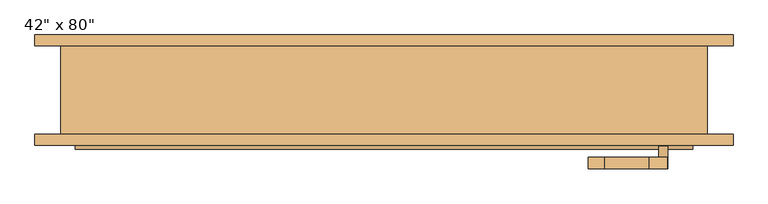
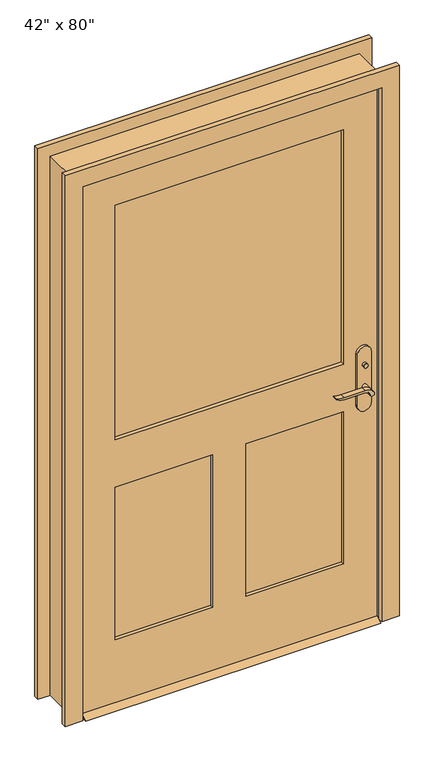
"""IFC4 building model written with IfcOpenShell, lengths in millimetres: door geometry."""

from ifc_helpers import new_model, si_unit, point, frame, frame_2d, origin, place, context, project, spatial, polyline, circle_curve, trimmed, segment, composite_curve, outline, extrude, faceted_brep, source, transform, mapped, element, save


def door_f970b2d0(model_context):
    return source(origin(), model_context, "Body", "SolidModel", [
        extrude(outline(polyline([(-38.1, 12.7), (-12.7, 0.0), (-98.425, 0.0), (-73.025, 12.7), (-38.1, 12.7)])), frame((-533.4, 0.0, 0.0), z_axis=(1.0, 0.0, 0.0), x_axis=(0.0, 1.0, 0.0)), (0.0, 0.0, 1.0), 1066.8),
        extrude(outline(polyline([(487.6, -18.1), (487.6, -28.1), (477.6, -28.1), (477.6, -18.1), (487.6, -18.1)])), frame((0.0, 0.0, 981.9), z_axis=(0.0, 0.0, 1.0), x_axis=(1.0, 0.0, 0.0)), (0.0, 0.0, 1.0), 30.0),
        extrude(outline(composite_curve([segment(trimmed(circle_curve(frame_2d((996.9, 482.6)), 8.0), [point((996.9, 474.6))], [point((996.9, 490.6))], False, "CARTESIAN"), True, "CONTINUOUS"), segment(trimmed(circle_curve(frame_2d((996.9, 482.6)), 8.0), [point((996.9, 490.6))], [point((996.9, 474.6))], False, "CARTESIAN"), True, "CONTINUOUS")], self_intersect=False)), frame((0.0, -93.025, 0.0), z_axis=(0.0, 1.0, 0.0), x_axis=(0.0, 0.0, 1.0)), (0.0, 0.0, 1.0), 10.0),
        extrude(outline(composite_curve([segment(trimmed(circle_curve(frame_2d((897.1555521, 458.9324871)), 37.2832219), [point((919.0523287, 489.1081363))], [point((934.4, 457.2325667))], False, "CARTESIAN"), True, "CONTINUOUS"), segment(polyline([(934.4, 457.2325667), (934.4, 380.9564091)]), True, "CONTINUOUS"), segment(trimmed(circle_curve(frame_2d((1017.6850638, 381.0227909)), 83.2850902), [point((934.4, 380.9564091))], [point((939.4, 352.6))], True, "CARTESIAN"), True, "CONTINUOUS"), segment(polyline([(939.4, 352.6), (936.6135558, 352.6)]), True, "CONTINUOUS"), segment(trimmed(circle_curve(frame_2d((986.6709207, 384.5396612)), 59.3791355), [point((936.6135558, 352.6))], [point((927.4, 380.9564091))], False, "CARTESIAN"), True, "CONTINUOUS"), segment(polyline([(927.4, 380.9564091), (927.4, 457.2138099)]), True, "CONTINUOUS"), segment(trimmed(circle_curve(frame_2d((909.2738613, 457.2138099)), 18.1261387), [point((927.4, 457.2138099))], [point((914.4, 474.6))], True, "CARTESIAN"), True, "CONTINUOUS"), segment(trimmed(circle_curve(frame_2d((914.4, 482.6)), 8.0), [point((914.4, 474.6))], [point((919.0523287, 489.1081363))], False, "CARTESIAN"), True, "CONTINUOUS")], self_intersect=False)), frame((0.0, 1.9, 0.0), z_axis=(0.0, 1.0, 0.0), x_axis=(0.0, 0.0, 1.0)), (0.0, 0.0, 1.0), 20.0),
        extrude(outline(composite_curve([segment(trimmed(circle_curve(frame_2d((914.4, 482.6)), 8.0), [point((914.3999903, 474.6))], [point((919.0523287, 489.1081363))], False, "CARTESIAN"), True, "CONTINUOUS"), segment(trimmed(circle_curve(frame_2d((897.1555521, 458.9324871)), 37.2832219), [point((919.0523287, 489.1081363))], [point((934.4, 457.2325667))], False, "CARTESIAN"), True, "CONTINUOUS"), segment(polyline([(934.4, 457.2325667), (934.4, 380.9564091)]), True, "CONTINUOUS"), segment(trimmed(circle_curve(frame_2d((1017.6850638, 381.0227909)), 83.2850902), [point((934.4, 380.9564091))], [point((939.4, 352.6))], True, "CARTESIAN"), True, "CONTINUOUS"), segment(polyline([(939.4, 352.6), (936.6135558, 352.6)]), True, "CONTINUOUS"), segment(trimmed(circle_curve(frame_2d((986.6709207, 384.5396612)), 59.3791355), [point((936.6135558, 352.6))], [point((927.4, 380.9564091))], False, "CARTESIAN"), True, "CONTINUOUS"), segment(polyline([(927.4, 380.9564091), (927.4, 457.2138122)]), True, "CONTINUOUS"), segment(trimmed(circle_curve(frame_2d((909.2738682, 457.2138122)), 18.1261318), [point((927.4, 457.2138122))], [point((914.3999903, 474.6))], True, "CARTESIAN"), True, "CONTINUOUS")], self_intersect=False)), frame((0.0, -133.025, 0.0), z_axis=(0.0, 1.0, 0.0), x_axis=(0.0, 0.0, 1.0)), (0.0, 0.0, 1.0), 20.0),
        extrude(outline(composite_curve([segment(trimmed(circle_curve(frame_2d((914.4, 482.6)), 8.0), [point((914.4, 474.6))], [point((914.4, 490.6))], False, "CARTESIAN"), True, "CONTINUOUS"), segment(trimmed(circle_curve(frame_2d((914.4, 482.6)), 8.0), [point((914.4, 490.6))], [point((914.4, 474.6))], False, "CARTESIAN"), True, "CONTINUOUS")], self_intersect=False)), frame((0.0, -28.1, 0.0), z_axis=(0.0, 1.0, 0.0), x_axis=(0.0, 0.0, 1.0)), (0.0, 0.0, 1.0), 30.0),
        extrude(outline(composite_curve([segment(trimmed(circle_curve(frame_2d((914.4, 482.6)), 8.0), [point((914.4, 474.6))], [point((914.4, 490.6))], False, "CARTESIAN"), True, "CONTINUOUS"), segment(trimmed(circle_curve(frame_2d((914.4, 482.6)), 8.0), [point((914.4, 490.6))], [point((914.4, 474.6))], False, "CARTESIAN"), True, "CONTINUOUS")], self_intersect=False)), frame((0.0, -113.025, 0.0), z_axis=(0.0, 1.0, 0.0), x_axis=(0.0, 0.0, 1.0)), (0.0, 0.0, 1.0), 30.0),
        extrude(outline(composite_curve([segment(polyline([(844.4, 507.6), (1039.4, 507.6)]), True, "CONTINUOUS"), segment(trimmed(circle_curve(frame_2d((1039.4, 482.6)), 25.0), [point((1039.4, 507.6))], [point((1039.4, 457.6))], False, "CARTESIAN"), True, "CONTINUOUS"), segment(polyline([(1039.4, 457.6), (844.4, 457.6)]), True, "CONTINUOUS"), segment(trimmed(circle_curve(frame_2d((844.4, 482.6)), 25.0), [point((844.4, 457.6))], [point((844.4, 507.6))], False, "CARTESIAN"), True, "CONTINUOUS")], self_intersect=False)), frame((0.0, -38.1, 0.0), z_axis=(0.0, 1.0, 0.0), x_axis=(0.0, 0.0, 1.0)), (0.0, 0.0, 1.0), 10.0),
        extrude(outline(composite_curve([segment(polyline([(844.4, 507.6), (1039.4, 507.6)]), True, "CONTINUOUS"), segment(trimmed(circle_curve(frame_2d((1039.4, 482.6)), 25.0), [point((1039.4, 507.6))], [point((1039.4, 457.6))], False, "CARTESIAN"), True, "CONTINUOUS"), segment(polyline([(1039.4, 457.6), (844.4, 457.6)]), True, "CONTINUOUS"), segment(trimmed(circle_curve(frame_2d((844.4, 482.6)), 25.0), [point((844.4, 457.6))], [point((844.4, 507.6))], False, "CARTESIAN"), True, "CONTINUOUS")], self_intersect=False)), frame((0.0, -83.025, 0.0), z_axis=(0.0, 1.0, 0.0), x_axis=(0.0, 0.0, 1.0)), (0.0, 0.0, 1.0), 10.0),
        extrude(outline(polyline([(2032.0, -533.4), (12.7, -533.4), (12.7, 533.4), (2032.0, 533.4), (2032.0, -533.4)]), holes=[polyline([(1016.0, -412.75), (1911.35, -412.75), (1911.35, 412.75), (1016.0, 412.75), (1016.0, -412.75)]), polyline([(835.025, -60.325), (254.0, -60.325), (254.0, -412.75), (835.025, -412.75), (835.025, -60.325)]), polyline([(835.025, 412.75), (254.0, 412.75), (254.0, 60.325), (835.025, 60.325), (835.025, 412.75)])]), frame((0.0, -73.025, 0.0), z_axis=(0.0, 1.0, 0.0), x_axis=(0.0, 0.0, 1.0)), (0.0, 0.0, 1.0), 34.925),
        faceted_brep([(558.8, -73.025, 0.0), (533.4, -73.025, 0.0), (533.4, -38.1, 0.0), (520.7, -38.1, 0.0), (520.7, -3.175, 0.0), (533.4, -3.175, 0.0), (533.4, 79.375, 0.0), (558.8, 79.375, 0.0), (558.8, 79.375, 2057.4), (558.8, -73.025, 2057.4), (533.4, 79.375, 2032.0), (-533.4, 79.375, 2032.0), (-533.4, 79.375, 0.0), (-558.8, 79.375, 0.0), (-558.8, 79.375, 2057.4), (533.4, -3.175, 2032.0), (520.7, -3.175, 2019.3), (-520.7, -3.175, 2019.3), (-520.7, -3.175, 0.0), (-533.4, -3.175, 0.0), (-533.4, -3.175, 2032.0), (520.7, -38.1, 2019.3), (533.4, -38.1, 2032.0), (-533.4, -38.1, 2032.0), (-533.4, -38.1, 0.0), (-520.7, -38.1, 0.0), (-520.7, -38.1, 2019.3), (533.4, -73.025, 2032.0), (-558.8, -73.025, 2057.4), (-558.8, -73.025, 0.0), (-533.4, -73.025, 0.0), (-533.4, -73.025, 2032.0)], [[[0, 1, 2, 3, 4, 5, 6, 7]], [[7, 8, 9, 0]], [[6, 10, 11, 12, 13, 14, 8, 7]], [[5, 15, 10, 6]], [[4, 16, 17, 18, 19, 20, 15, 5]], [[3, 21, 16, 4]], [[2, 22, 23, 24, 25, 26, 21, 3]], [[1, 27, 22, 2]], [[0, 9, 28, 29, 30, 31, 27, 1]], [[8, 14, 28, 9]], [[15, 20, 11, 10]], [[21, 26, 17, 16]], [[27, 31, 23, 22]], [[29, 13, 12, 19, 18, 25, 24, 30]], [[14, 13, 29, 28]], [[20, 19, 12, 11]], [[26, 25, 18, 17]], [[31, 30, 24, 23]]]),
        extrude(outline(polyline([(-60.325, -49.7416667), (-60.325, -61.3833333), (-412.75, -61.3833333), (-412.75, -49.7416667), (-60.325, -49.7416667)])), frame((0.0, 0.0, 254.0), z_axis=(0.0, 0.0, 1.0), x_axis=(1.0, 0.0, 0.0)), (0.0, 0.0, 1.0), 581.025),
        extrude(outline(polyline([(412.75, -49.7416667), (412.75, -61.3833333), (60.325, -61.3833333), (60.325, -49.7416667), (412.75, -49.7416667)])), frame((0.0, 0.0, 254.0), z_axis=(0.0, 0.0, 1.0), x_axis=(1.0, 0.0, 0.0)), (0.0, 0.0, 1.0), 581.025),
        extrude(outline(polyline([(412.75, -52.07), (412.75, -59.055), (-412.75, -59.055), (-412.75, -52.07), (412.75, -52.07)])), frame((0.0, 0.0, 1016.0), z_axis=(0.0, 0.0, 1.0), x_axis=(1.0, 0.0, 0.0)), (0.0, 0.0, 1.0), 895.35),
        extrude(outline(polyline([(0.0, -539.75), (2038.35, -539.75), (2038.35, 539.75), (0.0, 539.75), (0.0, 603.25), (2101.85, 603.25), (2101.85, -603.25), (0.0, -603.25), (0.0, -539.75)])), frame((0.0, 79.375, 0.0), z_axis=(0.0, 1.0, 0.0), x_axis=(0.0, 0.0, 1.0)), (0.0, 0.0, 1.0), 19.05),
        extrude(outline(polyline([(0.0, -539.75), (2038.35, -539.75), (2038.35, 539.75), (0.0, 539.75), (0.0, 603.25), (2101.85, 603.25), (2101.85, -603.25), (0.0, -603.25), (0.0, -539.75)])), frame((0.0, -92.075, 0.0), z_axis=(0.0, 1.0, 0.0), x_axis=(0.0, 0.0, 1.0)), (0.0, 0.0, 1.0), 19.05),
    ])


if __name__ == "__main__":
    model = new_model("IFC4")
    model_context = context("Model", 3, world=origin())
    ifc_project = project(units=[si_unit("LENGTHUNIT", "METRE", prefix="MILLI")], contexts=[model_context])
    site = spatial("IfcSite", under=ifc_project)
    building = spatial("IfcBuilding", under=site)
    placement = place(None, origin())
    door_shape = door_f970b2d0(model_context)
    element("IfcDoor", 1, ObjectType="42\" x 80\"", at=placement, inside=building, context=model_context, shape_type="MappedRepresentation", body=[
        mapped(door_shape, transform((0.0, 0.0, 0.0), x_axis=(1.0, 0.0, 0.0), y_axis=(0.0, 1.0, 0.0), z_axis=(0.0, 0.0, 1.0))),
    ])
    save(model, "model.ifc")

# Revit data of these elements
# Type "42\" x 80\""
#   Type Mark = "9"
#   Assembly Code = "B2030100"
#   Analytic Construction = "French door, wood frame with single glass"
#   Top Rail = 0' - 4 3/4"
#   Threshold Offset [instance default] = 0' - 0 1/2"
#   Thickness = 0' - 1 3/8"
#   Thermal Resistance (R) = 1.0696 (h·ft²·°F)/BTU
#   Swing Angle [instance default] = 90.00°
#   Stiles = 0' - 4 3/4"
#   Rough Width = 3' - 8"
#   Rough Height = 6' - 9"
#   Lock Rail = 0' - 7 1/8"
#   Height = 6' - 8"
#   Width = 3' - 6"
#   Heat Transfer Coefficient (U) = 0.9350 BTU/(h·ft²·°F)
#   Door Offset [instance default] = 0' - 0"
#   Bottom Rail = 0' - 9 1/2"
#   Threshold [instance default] = yes
#   Function = 1
#   Exterior Trim [instance default] = yes
#   Trim Material = Cherry
#   Threshold Material = Cherry
#   Panel Material = Cherry
#   Glazing = Glass
#   Frame Material = Cherry
#   Door Handle Material = Aluminum
#   Visual Light Transmittance = 0
#   Solar Heat Gain Coefficient = 0
#   Wall Closure = (empty or 0)
#   Construction Type = (empty or 0)
# Element 1 (IfcDoor, "42\" x 80\"")
#   Materials on its faces: "Cherry", "Aluminum", "Glass"
# Materials
#   "Cherry": class "Wood", colour RGB 226 177 128, transparency 0, Description = "Prunus Serotina", Cost = 0
#   "Glass": class "Glass", colour RGB 0 128 192, transparency 0.75, Description = "Soda Lime Glass", Cost = 0
#   "Aluminum": class "Metal", colour RGB 247 247 247, transparency 0, Description = "Aluminum 6061", Cost = 0
